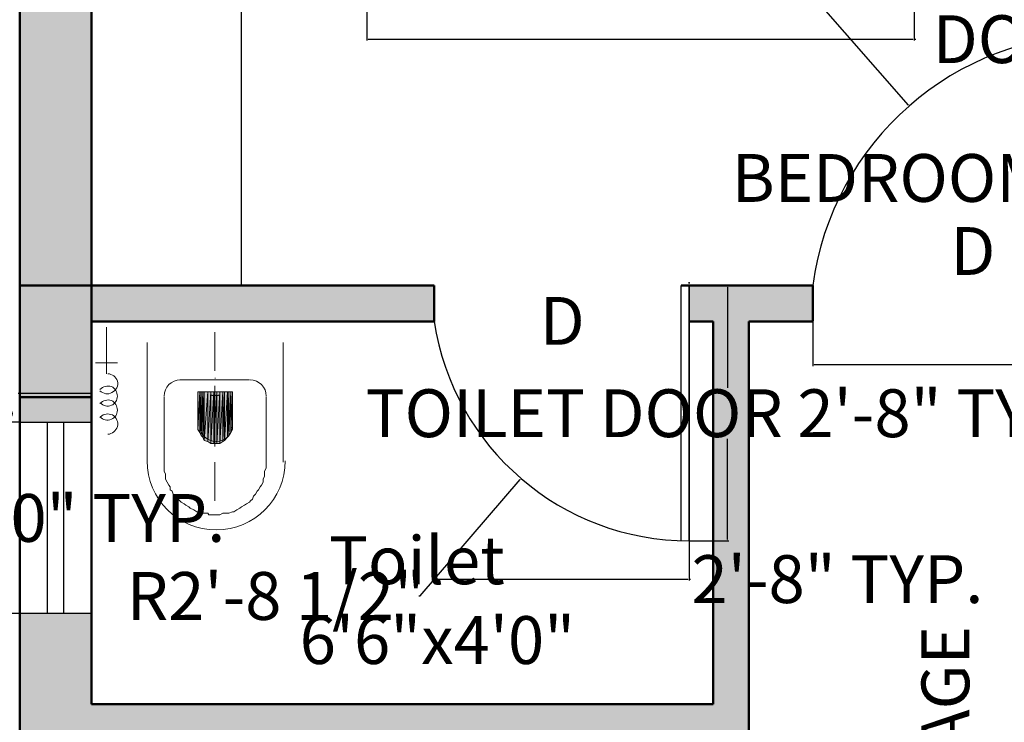
# Model space of a CAD drawing. Units: inches. Extents: x 1601 to 2080, y 5000 to 5589.
# Tile 8 of 11: x 1688 to 1812, y 5259 to 5348. Entities that reach past the tile are written whole.
import ezdxf

# ---------------------------------------------------------------- set-up
doc = ezdxf.new("R2010")
doc.units = ezdxf.units.IN
doc.header["$MEASUREMENT"] = 0
for name, color, linetype, lineweight in [('A-ANNO-DIMS', 2, 'Continuous', 18), ('A-ANNO-TEXT', 7, 'Continuous', 25), ('A-AREA-IDEN', 7, 'Continuous', 25), ('A-COLS', 7, 'Continuous', 50), ('A-COLS-PATT', 18, 'Continuous', 13), ('A-DOOR', 3, 'Continuous', 25), ('A-FLOR-CASE', 8, 'Continuous', 25), ('A-FLOR-FIXT', 7, 'Continuous', 18), ('A-FLOR-PATT', 8, 'Continuous', 13), ('A-GLAZ', 4, 'Continuous', 25), ('A-WALL', 7, 'Continuous', 50), ('A-WALL-PATT', 241, 'Continuous', 13)]:
    doc.layers.add(name, color=color, linetype=linetype, lineweight=lineweight)
doc.styles.get("Standard").update_dxf_attribs({"font": 'arial.ttf'})
doc.dimstyles.get("Standard").update_dxf_attribs({"dimtxt": 6, "dimasz": 0.18, "dimexe": 0.18, "dimexo": 0.0625, "dimgap": 0.09, "dimtad": 0, "dimtih": 1, "dimtoh": 1, "dimdec": 1, "dimzin": 0, "dimdsep": 46, "dimlunit": 3, "dimtxsty": 'Standard', "dimcen": 0.09, "dimadec": 0, "dimazin": 0, "dimtfac": 1, "dimtdec": 1, "dimtofl": 0, "dimtmove": 0, "dimatfit": 3, "dimfxl": 1, "dimtolj": 1, "dimtzin": 0, "dimarcsym": 0})

# ---------------------------------------------------------------- blocks, each defined once
blk = doc.blocks.new('WC')
h = blk.add_hatch(color=256)
h.paths.add_polyline_path([(12.84, 17.3), (12.84, 12.59), (13.07, 17.3)])
h.paths.add_polyline_path([(12.84, 12.59), (13.07, 17.3), (13.07, 12.21)])
h = blk.add_hatch(color=256)
h.paths.add_polyline_path([(13.07, 17.3), (13.07, 12.21), (13.22, 17.3)])
h.paths.add_polyline_path([(13.07, 12.21), (13.22, 17.3), (13.22, 11.83)])
h = blk.add_hatch(color=256)
h.paths.add_polyline_path([(13.22, 17.3), (13.22, 11.83), (13.45, 17.3)])
h.paths.add_polyline_path([(13.22, 11.83), (13.45, 17.3), (13.45, 11.61)])
h = blk.add_hatch(color=256)
h.paths.add_polyline_path([(13.45, 17.3), (13.45, 11.61), (13.6, 17.3)])
h.paths.add_polyline_path([(13.45, 11.61), (13.6, 17.3), (13.6, 11.23)])
h = blk.add_hatch(color=256)
h.paths.add_polyline_path([(13.6, 17.3), (13.6, 11.23), (14.06, 17.3)])
h.paths.add_polyline_path([(13.6, 11.23), (14.06, 17.3), (14.06, 11.08)])
h = blk.add_hatch(color=256)
h.paths.add_polyline_path([(14.06, 17.3), (14.06, 11.08), (14.44, 17.3)])
h.paths.add_polyline_path([(14.06, 11.08), (14.44, 17.3), (14.44, 10.85)])
h = blk.add_hatch(color=256)
h.paths.add_polyline_path([(14.44, 17.3), (14.44, 10.85), (14.81, 17.3)])
h.paths.add_polyline_path([(14.44, 10.85), (14.81, 17.3), (14.81, 10.85)])
h = blk.add_hatch(color=256)
h.paths.add_polyline_path([(14.81, 17.3), (14.81, 10.85), (15.19, 17.3)])
h.paths.add_polyline_path([(14.81, 10.85), (15.19, 17.3), (15.19, 10.85)])
h = blk.add_hatch(color=256)
h.paths.add_polyline_path([(15.19, 17.3), (15.19, 10.85), (15.57, 17.3)])
h.paths.add_polyline_path([(15.19, 10.85), (15.57, 17.3), (15.57, 10.85)])
h = blk.add_hatch(color=256)
h.paths.add_polyline_path([(15.57, 17.3), (15.57, 10.85), (15.95, 17.3)])
h.paths.add_polyline_path([(15.57, 10.85), (15.95, 17.3), (15.95, 11.08)])
h = blk.add_hatch(color=256)
h.paths.add_polyline_path([(15.95, 17.3), (15.95, 11.08), (16.18, 17.3)])
h.paths.add_polyline_path([(15.95, 11.08), (16.18, 17.3), (16.18, 11.23)])
h = blk.add_hatch(color=256)
h.paths.add_polyline_path([(16.18, 17.3), (16.18, 11.23), (16.56, 17.3)])
h.paths.add_polyline_path([(16.18, 11.23), (16.56, 17.3), (16.56, 11.61)])
h = blk.add_hatch(color=256)
h.paths.add_polyline_path([(16.56, 17.3), (16.56, 11.61), (16.71, 17.3)])
h.paths.add_polyline_path([(16.56, 11.61), (16.71, 17.3), (16.71, 11.83)])
h = blk.add_hatch(color=256)
h.paths.add_polyline_path([(16.71, 17.3), (16.71, 11.83), (16.94, 17.3)])
h.paths.add_polyline_path([(16.71, 11.83), (16.94, 17.3), (16.94, 12.21)])
h = blk.add_hatch(color=256)
h.paths.add_polyline_path([(16.94, 17.3), (16.94, 12.21), (17.17, 17.3)])
h.paths.add_polyline_path([(16.94, 12.21), (17.17, 17.3), (17.17, 12.59)])
h.paths.add_polyline_path([(17.17, 17.3), (17.17, 12.59), (17.17, 12.97)])
for points in [[(1.37, 25.41), (1.37, 19.57), (1.37, 19.57)], [(14.97, 24.81), (14.97, 19.95), (14.97, 19.95)], [(6.47, 23.52), (6.47, 8.5), (6.47, 8.5)], [(23.54, 23.52), (23.54, 8.5), (23.54, 8.5)], [(2.73, 20.94), (0, 20.94), (0, 20.94)], [(19.29, 18.81), (10.57, 18.81), (10.57, 18.81)], [(14.97, 19.04), (15.04, 19.04), (15.04, 19.04)], [(14.97, 18.05), (14.97, 10.47), (14.97, 10.47)], [(8.59, 16.69), (8.59, 9.48), (8.59, 9.48)], [(17.17, 17.3), (12.84, 17.3), (12.84, 17.3)], [(12.84, 17.3), (12.84, 12.97), (12.84, 12.97)], [(14.59, 16.84), (14.59, 16.92), (14.59, 16.92)], [(14.97, 16.84), (14.81, 16.84), (14.59, 16.84)], [(14.97, 16.84), (15.04, 16.92), (15.04, 16.92)], [(15.42, 16.84), (15.19, 16.84), (14.97, 16.84)], [(15.42, 16.84), (15.42, 16.92), (15.42, 16.92)], [(17.17, 17.3), (17.17, 12.97), (17.17, 12.97)], [(21.41, 16.69), (21.41, 9.48), (21.41, 9.48)], [(21.41, 9.48), (21.41, 8.72), (21.41, 8.12), (21.41, 7.74), (21.19, 7.36), (21.19, 6.98), (21.19, 6.75), (21.03, 6.37), (21.03, 5.99), (20.81, 5.61), (20.66, 5.39), (20.43, 5.01), (20.28, 4.85), (20.05, 4.48), (19.82, 4.25), (19.67, 3.87), (19.44, 3.64), (19.29, 3.49), (18.91, 3.26), (18.68, 3.11), (18.3, 2.88), (18.08, 2.73), (17.7, 2.5), (17.32, 2.28), (17.17, 2.28), (16.71, 2.12), (16.33, 2.12), (15.95, 2.12), (15.57, 1.9), (14.97, 1.9), (14.21, 1.9), (14.06, 2.12), (13.6, 2.12), (13.22, 2.12), (12.84, 2.28), (12.69, 2.28), (12.31, 2.5), (11.86, 2.73), (11.7, 2.88), (11.32, 3.11), (11.1, 3.26), (10.72, 3.49), (10.57, 3.64), (10.34, 3.87), (9.96, 4.25), (9.73, 4.48), (9.58, 4.85), (9.35, 5.01), (9.35, 5.39), (9.2, 5.61), (8.97, 5.99), (8.75, 6.37), (8.75, 6.75), (8.75, 6.98), (8.59, 7.36), (8.59, 7.74), (8.59, 8.12), (8.59, 8.72), (8.59, 9.48)], [(14.97, 8.5), (14.97, 3.64), (14.97, 3.64)]]:
    blk.add_lwpolyline(points)
for points in [[(12.84, 17.3), (12.84, 12.97)], [(12.84, 12.97), (12.84, 17.3), (12.84, 12.59)], [(12.84, 17.3), (12.84, 12.59), (13.07, 17.3)], [(12.84, 12.59), (13.07, 17.3), (13.07, 12.21)], [(13.07, 17.3), (13.07, 12.21), (13.22, 17.3)], [(13.07, 12.21), (13.22, 17.3), (13.22, 11.83)], [(13.22, 17.3), (13.22, 11.83), (13.45, 17.3)], [(13.22, 11.83), (13.45, 17.3), (13.45, 11.61)], [(13.45, 17.3), (13.45, 11.61), (13.6, 17.3)], [(13.45, 11.61), (13.6, 17.3), (13.6, 11.23)], [(13.6, 17.3), (13.6, 11.23), (14.06, 17.3)], [(13.6, 11.23), (14.06, 17.3), (14.06, 11.08)], [(14.06, 17.3), (14.06, 11.08), (14.44, 17.3)], [(14.06, 11.08), (14.44, 17.3), (14.44, 10.85)], [(14.44, 17.3), (14.44, 10.85), (14.81, 17.3)], [(14.44, 10.85), (14.81, 17.3), (14.81, 10.85)], [(14.81, 17.3), (14.81, 10.85), (15.19, 17.3)], [(14.81, 10.85), (15.19, 17.3), (15.19, 10.85)], [(15.19, 17.3), (15.19, 10.85), (15.57, 17.3)], [(15.19, 10.85), (15.57, 17.3), (15.57, 10.85)], [(15.57, 17.3), (15.57, 10.85), (15.95, 17.3)], [(15.57, 10.85), (15.95, 17.3), (15.95, 11.08)], [(15.95, 17.3), (15.95, 11.08), (16.18, 17.3)], [(15.95, 11.08), (16.18, 17.3), (16.18, 11.23)], [(16.18, 17.3), (16.18, 11.23), (16.56, 17.3)], [(16.18, 11.23), (16.56, 17.3), (16.56, 11.61)], [(16.56, 17.3), (16.56, 11.61), (16.71, 17.3)], [(16.56, 11.61), (16.71, 17.3), (16.71, 11.83)], [(16.71, 17.3), (16.71, 11.83), (16.94, 17.3)], [(16.71, 11.83), (16.94, 17.3), (16.94, 12.21)], [(16.94, 17.3), (16.94, 12.21), (17.17, 17.3)], [(16.94, 12.21), (17.17, 17.3), (17.17, 12.59)], [(17.17, 17.3), (17.17, 12.59), (17.17, 12.97)], [(17.17, 12.59), (17.17, 17.3), (17.17, 17.3)]]:
    blk.add_lwpolyline(points, close=True)
for points, knots in [([(0.53, 17.45), (0.91, 17.07), (1.59, 16.92), (2.05, 17.22), (2.05, 17.22), (2.58, 17.52), (2.88, 18.05), (2.73, 18.66), (2.73, 18.66), (2.58, 19.19), (2.05, 19.57), (1.52, 19.57)], [0, 0, 0, 0, 0.083333, 0.083333, 0.083333, 0.083334, 0.166667, 0.166667, 0.166667, 0.166668, 1, 1, 1, 1]), ([(0.61, 15.93), (0.91, 15.55), (1.52, 15.4), (1.97, 15.63), (1.97, 15.63), (2.43, 15.78), (2.73, 16.31), (2.73, 16.76), (2.73, 16.76), (2.73, 17.3), (2.43, 17.75), (1.97, 17.98), (1.97, 17.98), (1.44, 18.13), (0.91, 17.98), (0.53, 17.6)], [0, 0, 0, 0, 0.0625, 0.0625, 0.0625, 0.062501, 0.125, 0.125, 0.125, 0.125001, 0.1875, 0.1875, 0.1875, 0.187501, 1, 1, 1, 1]), ([(0.53, 14.19), (0.91, 13.81), (1.44, 13.65), (1.97, 13.88), (1.97, 13.88), (2.43, 14.03), (2.73, 14.49), (2.73, 15.02), (2.73, 15.02), (2.73, 15.55), (2.43, 16.01), (1.97, 16.23), (1.97, 16.23), (1.44, 16.39), (0.91, 16.23), (0.53, 15.85)], [0, 0, 0, 0, 0.0625, 0.0625, 0.0625, 0.062501, 0.125, 0.125, 0.125, 0.125001, 0.1875, 0.1875, 0.1875, 0.187501, 1, 1, 1, 1]), ([(1.52, 11.99), (2.05, 11.99), (2.58, 12.44), (2.73, 12.97), (2.73, 12.97), (2.88, 13.5), (2.58, 14.11), (2.12, 14.41), (2.12, 14.41), (1.59, 14.64), (0.99, 14.56), (0.61, 14.19)], [0, 0, 0, 0, 0.083333, 0.083333, 0.083333, 0.083334, 0.166667, 0.166667, 0.166667, 0.166668, 1, 1, 1, 1]), ([(13.07, 13.12), (13.07, 11.99), (13.98, 11.08), (15.12, 11.08), (15.12, 11.08), (16.26, 11.08), (17.17, 11.99), (17.17, 13.12)], [0, 0, 0, 0, 0.125, 0.125, 0.125, 0.125001, 1, 1, 1, 1]), ([(6.47, 8.65), (6.47, 3.87), (10.34, 0), (15.12, 0), (15.12, 0), (19.9, 0), (23.77, 3.87), (23.77, 8.65)], [0, 0, 0, 0, 0.125, 0.125, 0.125, 0.125001, 1, 1, 1, 1])]:
    blk.add_open_spline(points, degree=3, knots=knots)
for points in [[(10.64, 18.81), (9.5, 18.81), (8.59, 17.9), (8.59, 16.76)], [(21.41, 16.76), (21.41, 17.9), (20.5, 18.81), (19.37, 18.81)]]:
    blk.add_open_spline(points, degree=3)
blk = doc.blocks.new('DOOR-36IN')
for p, q in [((35, 36), (35, 0)), ((36, 0), (36, 36)), ((36, 36), (36, 0)), ((36, 0), (35, 0))]:
    blk.add_line(p, q)
blk.add_arc((36, -0.32), 36.32, 90, 172.3719)
blk = doc.blocks.new('DOOR-32IN')
for p, q in [((32, 32), (31, 32)), ((31, 0), (31, 32)), ((32, 32), (32, 0)), ((32, 0), (32, 32))]:
    blk.add_line(p, q)
blk.add_arc((32, 32.37), 32.37, 188.6501, 270)
blk = doc.blocks.new('VENT-24IN')
for p, q in [((0, 0), (0, 24)), ((0, 24), (9, 24)), ((3.5, 0), (3.5, 24)), ((5.5, 24), (5.5, 0)), ((9, 24), (9, 0)), ((9, 0), (0, 0))]:
    blk.add_line(p, q)
blk = doc.blocks.new('*D17')
at = {"layer": 'A-ANNO-DIMS', "color": 0, "lineweight": -2, "transparency": 16777216}
for p, q in [((1731.95, 5355.35), (1731.95, 5344.92)), ((1800.66, 5355.35), (1800.66, 5344.92)), ((1732.13, 5345.1), (1800.48, 5345.1)), ((1800.66, 5345.1), (1800.84, 5345.1))]:
    blk.add_line(p, q, dxfattribs=at)
at = {"layer": 'A-ANNO-DIMS', "color": 0, "transparency": 16777216}
for points in [[(1732.13, 5345.13), (1732.13, 5345.07), (1731.95, 5345.1)], [(1800.48, 5345.13), (1800.48, 5345.07), (1800.66, 5345.1)]]:
    blk.add_solid(points, dxfattribs=at)
at = {"layer": 'Defpoints', "color": 0, "transparency": 16777216}
for p in [(1731.95, 5355.41), (1800.66, 5355.41), (1800.66, 5345.1)]:
    blk.add_point(p, dxfattribs=at)
at = {"layer": 'A-ANNO-DIMS', "color": 0, "transparency": 16777216, "insert": (1854.24, 5345.1), "char_height": 6, "attachment_point": 5}
blk.add_mtext('\\A1;DOUBLE BED 5\'-8 1/2" TYP.', dxfattribs=at)
blk = doc.blocks.new('*D23')
at = {"layer": 'A-ANNO-DIMS', "color": 0, "lineweight": -2, "transparency": 16777216}
for p, q in [((1823.97, 5345.7), (1829.49, 5345.7)), ((1829.31, 5345.52), (1829.31, 5330.89)), ((1829.31, 5309.88), (1829.31, 5324.5)), ((1823.97, 5309.7), (1829.49, 5309.7))]:
    blk.add_line(p, q, dxfattribs=at)
at = {"layer": 'A-ANNO-DIMS', "color": 0, "transparency": 16777216}
for points in [[(1829.28, 5345.52), (1829.34, 5345.52), (1829.31, 5345.7)], [(1829.28, 5309.88), (1829.34, 5309.88), (1829.31, 5309.7)]]:
    blk.add_solid(points, dxfattribs=at)
at = {"layer": 'Defpoints', "color": 0, "transparency": 16777216}
for p in [(1823.91, 5345.7), (1829.31, 5345.7), (1823.91, 5309.7)]:
    blk.add_point(p, dxfattribs=at)
at = {"layer": 'A-ANNO-DIMS', "color": 0, "transparency": 16777216, "insert": (1829.31, 5327.7), "char_height": 6, "attachment_point": 5}
blk.add_mtext('\\A1;BEDROOM DOOR 3\'-0" TYP.', dxfattribs=at)
blk = doc.blocks.new('*D24')
at = {"layer": 'A-ANNO-DIMS', "color": 0, "lineweight": -2, "transparency": 16777216}
for p, q in [((1787.91, 5309.63), (1787.91, 5304.12)), ((1823.91, 5309.63), (1823.91, 5304.12)), ((1788.09, 5304.3), (1823.73, 5304.3)), ((1823.91, 5304.3), (1824.09, 5304.3))]:
    blk.add_line(p, q, dxfattribs=at)
at = {"layer": 'A-ANNO-DIMS', "color": 0, "transparency": 16777216}
for points in [[(1788.09, 5304.33), (1788.09, 5304.27), (1787.91, 5304.3)], [(1823.73, 5304.33), (1823.73, 5304.27), (1823.91, 5304.3)]]:
    blk.add_solid(points, dxfattribs=at)
at = {"layer": 'Defpoints', "color": 0, "transparency": 16777216}
for p in [(1787.91, 5309.7), (1823.91, 5309.7), (1823.91, 5304.3)]:
    blk.add_point(p, dxfattribs=at)
at = {"layer": 'A-ANNO-DIMS', "color": 0, "transparency": 16777216, "insert": (1842.46, 5304.3), "char_height": 6, "attachment_point": 5}
blk.add_mtext('\\A1;3\'-0" TYP.', dxfattribs=at)
blk = doc.blocks.new('*D25')
at = {"layer": 'A-ANNO-DIMS', "color": 0, "lineweight": -2, "transparency": 16777216}
for p, q in [((1772.47, 5314.2), (1777.39, 5314.2)), ((1777.21, 5314.02), (1777.21, 5301.39)), ((1777.21, 5282.38), (1777.21, 5295)), ((1772.47, 5282.2), (1777.39, 5282.2))]:
    blk.add_line(p, q, dxfattribs=at)
at = {"layer": 'A-ANNO-DIMS', "color": 0, "transparency": 16777216}
for points in [[(1777.18, 5314.02), (1777.24, 5314.02), (1777.21, 5314.2)], [(1777.18, 5282.38), (1777.24, 5282.38), (1777.21, 5282.2)]]:
    blk.add_solid(points, dxfattribs=at)
at = {"layer": 'Defpoints', "color": 0, "transparency": 16777216}
for p in [(1772.41, 5314.2), (1777.21, 5314.2), (1772.41, 5282.2)]:
    blk.add_point(p, dxfattribs=at)
at = {"layer": 'A-ANNO-DIMS', "color": 0, "transparency": 16777216, "insert": (1777.21, 5298.2), "char_height": 6, "attachment_point": 5}
blk.add_mtext('\\A1;TOILET DOOR 2\'-8" TYP.', dxfattribs=at)
blk = doc.blocks.new('*D26')
at = {"layer": 'A-ANNO-DIMS', "color": 0, "lineweight": -2, "transparency": 16777216}
for p, q in [((1740.41, 5282.13), (1740.41, 5277.22)), ((1772.41, 5282.13), (1772.41, 5277.22)), ((1740.59, 5277.4), (1772.23, 5277.4)), ((1772.41, 5277.4), (1772.59, 5277.4))]:
    blk.add_line(p, q, dxfattribs=at)
at = {"layer": 'A-ANNO-DIMS', "color": 0, "transparency": 16777216}
for points in [[(1740.59, 5277.43), (1740.59, 5277.37), (1740.41, 5277.4)], [(1772.23, 5277.43), (1772.23, 5277.37), (1772.41, 5277.4)]]:
    blk.add_solid(points, dxfattribs=at)
at = {"layer": 'Defpoints', "color": 0, "transparency": 16777216}
for p in [(1740.41, 5282.2), (1772.41, 5282.2), (1772.41, 5277.4)]:
    blk.add_point(p, dxfattribs=at)
at = {"layer": 'A-ANNO-DIMS', "color": 0, "transparency": 16777216, "insert": (1791.02, 5277.4), "char_height": 6, "attachment_point": 5}
blk.add_mtext('\\A1;2\'-8" TYP.', dxfattribs=at)
blk = doc.blocks.new('*D31')
at = {"layer": 'A-ANNO-DIMS', "color": 0, "lineweight": -2, "transparency": 16777216}
for p, q in [((1688.35, 5297.07), (1684.63, 5297.07)), ((1684.81, 5296.89), (1684.81, 5288.22)), ((1684.81, 5273.25), (1684.81, 5281.92)), ((1688.35, 5273.07), (1684.63, 5273.07))]:
    blk.add_line(p, q, dxfattribs=at)
at = {"layer": 'A-ANNO-DIMS', "color": 0, "transparency": 16777216}
for points in [[(1684.78, 5296.89), (1684.84, 5296.89), (1684.81, 5297.07)], [(1684.78, 5273.25), (1684.84, 5273.25), (1684.81, 5273.07)]]:
    blk.add_solid(points, dxfattribs=at)
at = {"layer": 'Defpoints', "color": 0, "transparency": 16777216}
for p in [(1688.41, 5297.07), (1684.81, 5273.07), (1688.41, 5273.07)]:
    blk.add_point(p, dxfattribs=at)
at = {"layer": 'A-ANNO-DIMS', "color": 0, "transparency": 16777216, "insert": (1684.81, 5285.07), "char_height": 6, "attachment_point": 5}
blk.add_mtext('\\A1;VENT 2\'-0" TYP.', dxfattribs=at)
blk = doc.blocks.new('*D32')
at = {"layer": 'A-ANNO-DIMS', "color": 0, "lineweight": -2, "transparency": 16777216}
for p, q in [((1688.41, 5300.67), (1688.23, 5300.67)), ((1688.41, 5297.13), (1688.41, 5300.85)), ((1697.23, 5300.67), (1688.59, 5300.67)), ((1697.41, 5297.13), (1697.41, 5300.85))]:
    blk.add_line(p, q, dxfattribs=at)
at = {"layer": 'A-ANNO-DIMS', "color": 0, "transparency": 16777216}
for points in [[(1688.59, 5300.7), (1688.59, 5300.64), (1688.41, 5300.67)], [(1697.23, 5300.7), (1697.23, 5300.64), (1697.41, 5300.67)]]:
    blk.add_solid(points, dxfattribs=at)
at = {"layer": 'Defpoints', "color": 0, "transparency": 16777216}
for p in [(1688.41, 5300.67), (1688.41, 5297.07), (1697.41, 5297.07)]:
    blk.add_point(p, dxfattribs=at)
at = {"layer": 'A-ANNO-DIMS', "color": 0, "transparency": 16777216, "insert": (1669.85, 5300.67), "char_height": 6, "attachment_point": 5}
blk.add_mtext('\\A1;0\'-9" TYP.', dxfattribs=at)
blk = doc.blocks.new('*D60')
at = {"layer": 'A-ANNO-DIMS', "color": 0, "lineweight": -2, "transparency": 16777216}
for p, q in [((1785.46, 5353.11), (1785.64, 5353.11)), ((1785.64, 5353.11), (1799.87, 5336.85)), ((1823.82, 5309.37), (1824, 5309.37)), ((1823.91, 5309.28), (1823.91, 5309.46))]:
    blk.add_line(p, q, dxfattribs=at)
at = {"layer": 'A-ANNO-DIMS', "color": 0, "transparency": 16777216}
blk.add_solid([(1799.89, 5336.86), (1799.85, 5336.83), (1799.99, 5336.71)], dxfattribs=at)
at = {"layer": 'Defpoints', "color": 0, "transparency": 16777216}
for p in [(1799.99, 5336.71), (1823.91, 5309.37)]:
    blk.add_point(p, dxfattribs=at)
at = {"layer": 'A-ANNO-DIMS', "color": 0, "transparency": 16777216, "insert": (1767.53, 5353.11), "char_height": 6, "attachment_point": 5}
blk.add_mtext('\\A1;R3\'-0 1/2"', dxfattribs=at)
blk = doc.blocks.new('*D61')
at = {"layer": 'A-ANNO-DIMS', "color": 0, "lineweight": -2, "transparency": 16777216}
for p, q in [((1772.32, 5314.56), (1772.5, 5314.56)), ((1772.41, 5314.47), (1772.41, 5314.65)), ((1738.65, 5275.29), (1751.19, 5289.88)), ((1738.47, 5275.29), (1738.65, 5275.29))]:
    blk.add_line(p, q, dxfattribs=at)
at = {"layer": 'A-ANNO-DIMS', "color": 0, "transparency": 16777216}
blk.add_solid([(1751.17, 5289.9), (1751.22, 5289.86), (1751.31, 5290.02)], dxfattribs=at)
at = {"layer": 'Defpoints', "color": 0, "transparency": 16777216}
for p in [(1772.41, 5314.56), (1751.31, 5290.02)]:
    blk.add_point(p, dxfattribs=at)
at = {"layer": 'A-ANNO-DIMS', "color": 0, "transparency": 16777216, "insert": (1720.55, 5275.29), "char_height": 6, "attachment_point": 5}
blk.add_mtext('\\A1;R2\'-8 1/2"', dxfattribs=at)

msp = doc.modelspace()

# ---------------------------------------------------------------- hatches: boundary and pattern name
at = {"layer": 'A-COLS-PATT'}
h = msp.add_hatch(color=256, dxfattribs=at)
h.dxf.hatch_style = 1
h.paths.add_polyline_path([(1702.41, 5431.2), (1688.41, 5431.2), (1688.41, 5422.2), (1702.41, 5422.2)])
h.paths.add_polyline_path([(1836.17, 5431.2), (1822.17, 5431.2), (1822.17, 5422.2), (1836.17, 5422.2)])
h.paths.add_polyline_path([(1962.91, 5431.2), (1948.91, 5431.2), (1948.91, 5422.2), (1962.91, 5422.2)])
h.paths.add_polyline_path([(1697.41, 5314.2), (1688.41, 5314.2), (1688.41, 5300.2), (1697.41, 5300.2)])
h.paths.add_polyline_path([(1833.91, 5314.2), (1824.91, 5314.2), (1824.91, 5300.2), (1833.91, 5300.2)])
h.paths.add_polyline_path([(1962.91, 5314.2), (1953.91, 5314.2), (1953.91, 5300.2), (1962.91, 5300.2)])
h.paths.add_polyline_path([(1697.41, 5209.2), (1688.41, 5209.2), (1688.41, 5195.2), (1697.41, 5195.2)])
h.paths.add_polyline_path([(1833.91, 5209.2), (1824.91, 5209.2), (1824.91, 5195.2), (1833.91, 5195.2)])
h.paths.add_polyline_path([(1962.91, 5209.2), (1953.91, 5209.2), (1953.91, 5195.2), (1962.91, 5195.2)])
h.paths.add_polyline_path([(1697.41, 5083.7), (1688.41, 5083.7), (1688.41, 5069.7), (1697.41, 5069.7)])
h.paths.add_polyline_path([(1833.91, 5078.7), (1819.91, 5078.7), (1819.91, 5069.7), (1833.91, 5069.7)])
h.paths.add_polyline_path([(1962.91, 5078.7), (1948.91, 5078.7), (1948.91, 5069.7), (1962.91, 5069.7)])
at = {"layer": 'A-FLOR-PATT'}
h = msp.add_hatch(dxfattribs=at)
h.set_pattern_fill('ANGLE', color=256, scale=40)
h.set_pattern_definition([(0, (0, 0), (0, 11), [8, -3]), (90, (0, 0), (-11, 7e-16), [8, -3])])
h.paths.add_polyline_path([(2022.91, 5509.2), (1941.91, 5509.2), (1911.91, 5509.2), (1864.41, 5509.2), (1864.41, 5489.7), (1868.54, 5489.7, -0.022155), (1868.52, 5490.01, -1), (1875.53, 5490.01, -0.956651), (1868.54, 5489.7), (1864.41, 5489.7), (1864.41, 5470.2), (1794.41, 5470.2), (1794.41, 5431.2), (1811.95, 5431.2), (1911.91, 5431.2), (1941.91, 5431.2), (1942.91, 5431.2), (1945.91, 5431.2), (1948.91, 5431.2), (1962.91, 5431.2), (1962.91, 5415.29), (1962.91, 5385.29), (1962.91, 5384.29), (1962.91, 5381.29), (1962.91, 5333.29), (1962.91, 5069.7), (2022.91, 5069.7)])
h.paths.add_polyline_path([(2000.28, 5267.55), (2000.28, 5367.64), (1987.91, 5367.64), (1987.91, 5267.55)], flags=24)
h.paths.add_polyline_path([(1879.42, 5455.52), (1969.04, 5455.52), (1969.04, 5467.88), (1879.42, 5467.88)], flags=24)
at = {"layer": 'A-WALL-PATT'}
h = msp.add_hatch(color=256, dxfattribs=at)
h.dxf.hatch_style = 1
h.paths.add_polyline_path([(1763.95, 5431.2), (1702.41, 5431.2), (1702.41, 5422.2), (1763.95, 5422.2)])
h.paths.add_polyline_path([(1697.41, 5422.2), (1688.41, 5422.2), (1688.41, 5314.2), (1697.41, 5314.2)])
h.paths.add_polyline_path([(1740.41, 5314.2), (1697.41, 5314.2), (1697.41, 5309.7), (1740.41, 5309.7)], flags=17)
h.paths.add_polyline_path([(1822.17, 5431.2), (1811.95, 5431.2), (1811.95, 5422.2), (1822.17, 5422.2)])
h.paths.add_polyline_path([(1845.52, 5431.2), (1836.17, 5431.2), (1836.17, 5422.2), (1845.52, 5422.2)])
h.paths.add_polyline_path([(1910.91, 5431.2), (1881.52, 5431.2), (1881.52, 5422.2), (1910.91, 5422.2)])
h.paths.add_polyline_path([(1948.91, 5431.2), (1945.91, 5431.2), (1942.91, 5431.2), (1942.91, 5422.2), (1948.91, 5422.2)])
h.paths.add_polyline_path([(1962.91, 5422.2), (1953.91, 5422.2), (1953.91, 5416.29), (1962.91, 5416.29)])
h.paths.add_polyline_path([(1962.91, 5384.29), (1953.91, 5384.29), (1953.91, 5381.29), (1962.91, 5381.29)])
h.paths.add_polyline_path([(1962.91, 5333.29), (1953.91, 5333.29), (1953.91, 5314.2), (1962.91, 5314.2)])
h.paths.add_polyline_path([(1962.91, 5300.2), (1953.91, 5300.2), (1953.91, 5236.2), (1875.91, 5236.2), (1875.91, 5230.7), (1881.91, 5230.7), (1881.91, 5231.7), (1953.91, 5231.7), (1953.91, 5219.2), (1962.91, 5219.2)])
h.paths.add_polyline_path([(1962.91, 5185.2), (1953.91, 5185.2), (1953.91, 5183.7), (1881.91, 5183.7), (1881.91, 5184.7), (1875.91, 5184.7), (1875.91, 5183.7), (1875.91, 5179.2), (1953.91, 5179.2), (1953.91, 5172.6), (1962.91, 5172.6)])
h.paths.add_polyline_path([(1962.91, 5136.6), (1953.91, 5136.6), (1953.91, 5078.7), (1962.91, 5078.7)])
h.paths.add_polyline_path([(1948.91, 5078.7), (1833.91, 5078.7), (1833.91, 5069.7), (1948.91, 5069.7)])
h.paths.add_polyline_path([(1833.91, 5195.2), (1829.41, 5195.2), (1829.41, 5078.7), (1833.91, 5078.7)])
h.paths.add_polyline_path([(1819.91, 5078.7), (1813.58, 5078.7), (1813.58, 5069.7), (1819.91, 5069.7)])
h.paths.add_polyline_path([(1765.58, 5078.7), (1697.41, 5078.7), (1697.41, 5069.7), (1765.58, 5069.7)])
h.paths.add_polyline_path([(1697.41, 5195.2), (1688.41, 5195.2), (1688.41, 5083.7), (1697.41, 5083.7)])
h.paths.add_polyline_path([(1740.41, 5209.2), (1697.41, 5209.2), (1697.41, 5204.7), (1740.41, 5204.7)], flags=17)
h.paths.add_polyline_path([(1787.91, 5209.2), (1779.91, 5209.2), (1779.91, 5309.7), (1787.91, 5309.7), (1787.91, 5314.2), (1772.41, 5314.2), (1772.41, 5309.7), (1775.41, 5309.7), (1775.41, 5261.7), (1697.41, 5261.7), (1697.41, 5273.07), (1688.41, 5273.07), (1688.41, 5242.37), (1697.41, 5242.37), (1697.41, 5257.2), (1775.41, 5257.2), (1775.41, 5209.2), (1772.41, 5209.2), (1772.41, 5204.7), (1775.41, 5204.7), (1787.91, 5204.7)])
h.paths.add_polyline_path([(1697.41, 5218.37), (1688.41, 5218.37), (1688.41, 5209.2), (1697.41, 5209.2)], flags=17)
h.paths.add_polyline_path([(1833.91, 5422.2), (1829.41, 5422.2), (1829.41, 5314.2), (1833.91, 5314.2)])
h.paths.add_polyline_path([(1697.41, 5300.2), (1688.41, 5300.2), (1688.41, 5297.07), (1697.41, 5297.07)], flags=17)

# ---------------------------------------------------------------- linework, layer by layer
at = {"layer": 'A-COLS'}
for p, q in [((1688.41, 5314.2), (1688.41, 5300.2)), ((1697.41, 5300.2), (1697.41, 5314.2)), ((1688.41, 5300.2), (1697.41, 5300.2))]:
    msp.add_line(p, q, dxfattribs=at)
at = {"layer": 'A-FLOR-CASE'}
msp.add_line((1716.19, 5422.2), (1716.19, 5314.2), dxfattribs=at)
at = {"layer": 'A-WALL'}
for p, q in [((1688.41, 5431.2), (1688.41, 5069.7)), ((1697.41, 5422.2), (1697.41, 5261.7)), ((1688.41, 5314.2), (1740.41, 5314.2)), ((1740.41, 5314.2), (1740.41, 5309.7)), ((1771.41, 5314.2), (1787.91, 5314.2)), ((1775.41, 5314.2), (1772.41, 5314.2)), ((1787.91, 5309.7), (1787.91, 5314.2)), ((1697.41, 5309.7), (1740.41, 5309.7)), ((1772.41, 5309.7), (1775.41, 5309.7)), ((1775.41, 5309.7), (1775.41, 5261.7)), ((1779.91, 5309.7), (1779.91, 5209.2)), ((1779.91, 5309.7), (1787.91, 5309.7)), ((1697.41, 5261.7), (1775.41, 5261.7))]:
    msp.add_line(p, q, dxfattribs=at)

# ---------------------------------------------------------------- block references
at = {"layer": 'A-DOOR'}
for name, p in [('DOOR-36IN', (1787.91, 5309.7)), ('DOOR-32IN', (1740.41, 5282.2))]:
    msp.add_blockref(name, p, dxfattribs=at)
at = {"layer": 'A-FLOR-FIXT'}
msp.add_blockref('WC', (1697.94, 5283.57), dxfattribs=at)
at = {"layer": 'A-GLAZ', "rotation": 180}
msp.add_blockref('VENT-24IN', (1697.41, 5297.07), dxfattribs=at)

# ---------------------------------------------------------------- texts
at = {"layer": 'A-ANNO-TEXT', "char_height": 6, "attachment_point": 1}
for insert in [(1805.2, 5321.54), (1753.67, 5312.78)]:
    msp.add_mtext_dynamic_manual_height_columns('D ', width=9.7695, gutter_width=30, heights=[0], dxfattribs=dict(at, insert=insert))
at = {"layer": 'A-AREA-IDEN', "insert": (1723.54, 5282.76), "char_height": 6, "attachment_point": 1}
msp.add_mtext_dynamic_manual_height_columns('  Toilet\\P6\'6"x4\'0"', width=35.0416, gutter_width=30, heights=[0], dxfattribs=at)
at = {"layer": 'A-AREA-IDEN', "insert": (1801.56, 5236.17), "char_height": 6, "attachment_point": 1, "rotation": 90}
msp.add_mtext_dynamic_manual_height_columns('PASSAGE', width=39.5906, gutter_width=30, heights=[0], dxfattribs=at)

# ---------------------------------------------------------------- dimensions: what is measured, and where the dimension line sits
at = {"layer": 'A-ANNO-DIMS'}
for base, p1, p2, text, picture, middle in [((1800.66, 5345.1), (1731.95, 5355.41), (1800.66, 5355.41), 'DOUBLE BED <> TYP.', '*D17', (1854.24, 5345.1)), ((1823.91, 5304.3), (1787.91, 5309.7), (1823.91, 5309.7), '<> TYP.', '*D24', (1842.46, 5304.3)), ((1772.41, 5277.4), (1740.41, 5282.2), (1772.41, 5282.2), '<> TYP.', '*D26', (1791.02, 5277.4))]:
    dim = msp.add_linear_dim(base=base, p1=p1, p2=p2, text=text, dimstyle='Standard', override={"dimdec": 1, "dimlfac": 1, "dimrnd": 0, "dimzin": 1, "dimdsep": 46, "dimlunit": 4, "dimfrac": 2}, dxfattribs=at)
    dim.commit()
    dim.dimension.update_dxf_attribs({"geometry": picture, "text_midpoint": middle})
for center, mpoint, picture, middle in [((1823.91, 5309.37), (1799.99, 5336.71), '*D60', (1767.53, 5353.11)), ((1772.41, 5314.56), (1751.31, 5290.02), '*D61', (1720.55, 5275.29))]:
    dim = msp.add_radius_dim(center=center, mpoint=mpoint, dimstyle='Standard', override={"dimdec": 1, "dimlfac": 1, "dimrnd": 0, "dimzin": 1, "dimdsep": 46, "dimlunit": 4, "dimfrac": 2}, dxfattribs=at)
    dim.commit()
    dim.dimension.update_dxf_attribs({"geometry": picture, "text_midpoint": middle, "dimtype": 164})
for base, p1, p2, angle, text, picture, middle in [((1829.31, 5345.7), (1823.91, 5309.7), (1823.91, 5345.7), 90, 'BEDROOM DOOR <> TYP.', '*D23', (1829.31, 5327.7)), ((1777.21, 5314.2), (1772.41, 5282.2), (1772.41, 5314.2), 90, 'TOILET DOOR <> TYP.', '*D25', (1777.21, 5298.2)), ((1688.41, 5300.67), (1697.41, 5297.07), (1688.41, 5297.07), 180, '<> TYP.', '*D32', (1669.85, 5300.67)), ((1684.81, 5273.07), (1688.41, 5297.07), (1688.41, 5273.07), 270, 'VENT <> TYP.', '*D31', (1684.81, 5285.07))]:
    dim = msp.add_linear_dim(base=base, p1=p1, p2=p2, angle=angle, text=text, dimstyle='Standard', override={"dimdec": 1, "dimlfac": 1, "dimrnd": 0, "dimzin": 1, "dimdsep": 46, "dimlunit": 4, "dimfrac": 2}, dxfattribs=at)
    dim.commit()
    dim.dimension.update_dxf_attribs({"geometry": picture, "text_midpoint": middle})

doc.saveas('drawing.dxf')
